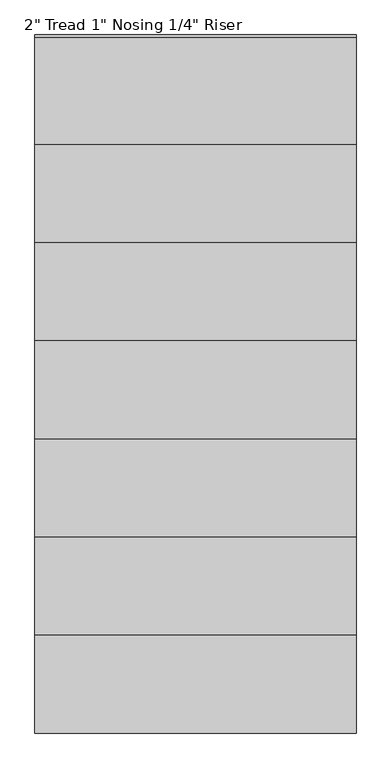
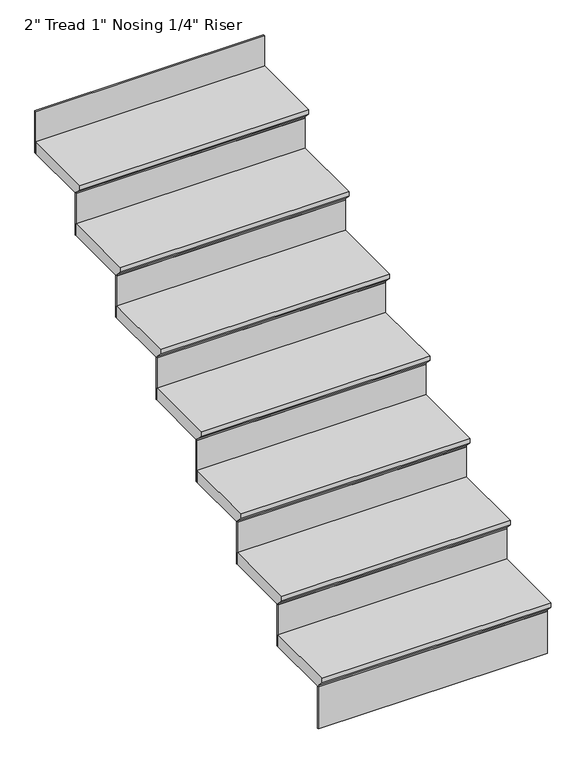
"""IFC4 building model written with IfcOpenShell, lengths in millimetres: stair flight geometry."""

from ifc_helpers import new_model, si_unit, frame, origin, place, context, project, spatial, polyline, outline, extrude, source, transform, mapped, element, save


def stair_flight_a0137449(model_context):
    return source(origin(), model_context, "Body", "SweptSolid", [
        extrude(outline(polyline([(-3589.3064015, 5765.8), (-3284.5064015, 5765.8), (-3284.5064015, 5715.0), (-3563.9064015, 5715.0), (-3563.9064015, 5721.35), (-3589.3064015, 5746.75), (-3589.3064015, 5765.8)])), frame((13296.7506237, 0.0, 0.0), z_axis=(1.0, 0.0, 0.0), x_axis=(0.0, 1.0, 0.0)), (0.0, 0.0, 1.0), 914.4),
        extrude(outline(polyline([(14211.1506237, -3557.5564015), (14211.1506237, -3563.9064015), (13296.7506237, -3563.9064015), (13296.7506237, -3557.5564015), (14211.1506237, -3557.5564015)])), frame((0.0, 0.0, 5537.2), z_axis=(0.0, 0.0, 1.0), x_axis=(1.0, 0.0, 0.0)), (0.0, 0.0, 1.0), 177.8),
        extrude(outline(polyline([(14211.1506237, -3278.1564015), (14211.1506237, -3284.5064015), (13296.7506237, -3284.5064015), (13296.7506237, -3278.1564015), (14211.1506237, -3278.1564015)])), frame((0.0, 0.0, 5715.0), z_axis=(0.0, 0.0, 1.0), x_axis=(1.0, 0.0, 0.0)), (0.0, 0.0, 1.0), 177.8),
        extrude(outline(polyline([(-3309.9064015, 5943.6), (-3005.1064015, 5943.6), (-3005.1064015, 5892.8), (-3284.5064015, 5892.8), (-3284.5064015, 5899.15), (-3309.9064015, 5924.55), (-3309.9064015, 5943.6)])), frame((13296.7506237, 0.0, 0.0), z_axis=(1.0, 0.0, 0.0), x_axis=(0.0, 1.0, 0.0)), (0.0, 0.0, 1.0), 914.4),
        extrude(outline(polyline([(14211.1506237, -2998.7564015), (14211.1506237, -3005.1064015), (13296.7506237, -3005.1064015), (13296.7506237, -2998.7564015), (14211.1506237, -2998.7564015)])), frame((0.0, 0.0, 5892.8), z_axis=(0.0, 0.0, 1.0), x_axis=(1.0, 0.0, 0.0)), (0.0, 0.0, 1.0), 177.8),
        extrude(outline(polyline([(-3030.5064015, 6121.4), (-2725.7064015, 6121.4), (-2725.7064015, 6070.6), (-3005.1064015, 6070.6), (-3005.1064015, 6076.95), (-3030.5064015, 6102.35), (-3030.5064015, 6121.4)])), frame((13296.7506237, 0.0, 0.0), z_axis=(1.0, 0.0, 0.0), x_axis=(0.0, 1.0, 0.0)), (0.0, 0.0, 1.0), 914.4),
        extrude(outline(polyline([(14211.1506237, -2719.3564015), (14211.1506237, -2725.7064015), (13296.7506237, -2725.7064015), (13296.7506237, -2719.3564015), (14211.1506237, -2719.3564015)])), frame((0.0, 0.0, 6070.6), z_axis=(0.0, 0.0, 1.0), x_axis=(1.0, 0.0, 0.0)), (0.0, 0.0, 1.0), 177.8),
        extrude(outline(polyline([(-2751.1064015, 6299.2), (-2446.3064015, 6299.2), (-2446.3064015, 6248.4), (-2725.7064015, 6248.4), (-2725.7064015, 6254.75), (-2751.1064015, 6280.15), (-2751.1064015, 6299.2)])), frame((13296.7506237, 0.0, 0.0), z_axis=(1.0, 0.0, 0.0), x_axis=(0.0, 1.0, 0.0)), (0.0, 0.0, 1.0), 914.4),
        extrude(outline(polyline([(14211.1506237, -2439.9564015), (14211.1506237, -2446.3064015), (13296.7506237, -2446.3064015), (13296.7506237, -2439.9564015), (14211.1506237, -2439.9564015)])), frame((0.0, 0.0, 6248.4), z_axis=(0.0, 0.0, 1.0), x_axis=(1.0, 0.0, 0.0)), (0.0, 0.0, 1.0), 177.8),
        extrude(outline(polyline([(-2471.7064015, 6477.0), (-2166.9064015, 6477.0), (-2166.9064015, 6426.2), (-2446.3064015, 6426.2), (-2446.3064015, 6432.55), (-2471.7064015, 6457.95), (-2471.7064015, 6477.0)])), frame((13296.7506237, 0.0, 0.0), z_axis=(1.0, 0.0, 0.0), x_axis=(0.0, 1.0, 0.0)), (0.0, 0.0, 1.0), 914.4),
        extrude(outline(polyline([(14211.1506237, -2160.5564015), (14211.1506237, -2166.9064015), (13296.7506237, -2166.9064015), (13296.7506237, -2160.5564015), (14211.1506237, -2160.5564015)])), frame((0.0, 0.0, 6426.2), z_axis=(0.0, 0.0, 1.0), x_axis=(1.0, 0.0, 0.0)), (0.0, 0.0, 1.0), 177.8),
        extrude(outline(polyline([(-2192.3064015, 6654.8), (-1887.5064015, 6654.8), (-1887.5064015, 6604.0), (-2166.9064015, 6604.0), (-2166.9064015, 6610.35), (-2192.3064015, 6635.75), (-2192.3064015, 6654.8)])), frame((13296.7506237, 0.0, 0.0), z_axis=(1.0, 0.0, 0.0), x_axis=(0.0, 1.0, 0.0)), (0.0, 0.0, 1.0), 914.4),
        extrude(outline(polyline([(14211.1506237, -1881.1564015), (14211.1506237, -1887.5064015), (13296.7506237, -1887.5064015), (13296.7506237, -1881.1564015), (14211.1506237, -1881.1564015)])), frame((0.0, 0.0, 6604.0), z_axis=(0.0, 0.0, 1.0), x_axis=(1.0, 0.0, 0.0)), (0.0, 0.0, 1.0), 177.8),
        extrude(outline(polyline([(14211.1506237, -1601.7564015), (14211.1506237, -1608.1064015), (13296.7506237, -1608.1064015), (13296.7506237, -1601.7564015), (14211.1506237, -1601.7564015)])), frame((0.0, 0.0, 6781.8), z_axis=(0.0, 0.0, 1.0), x_axis=(1.0, 0.0, 0.0)), (0.0, 0.0, 1.0), 177.8),
        extrude(outline(polyline([(-1912.9064015, 6832.6), (-1608.1064015, 6832.6), (-1608.1064015, 6781.8), (-1887.5064015, 6781.8), (-1887.5064015, 6788.15), (-1912.9064015, 6813.55), (-1912.9064015, 6832.6)])), frame((13296.7506237, 0.0, 0.0), z_axis=(1.0, 0.0, 0.0), x_axis=(0.0, 1.0, 0.0)), (0.0, 0.0, 1.0), 914.4),
    ])


if __name__ == "__main__":
    model = new_model("IFC4")
    model_context = context("Model", 3, world=origin())
    ifc_project = project(units=[si_unit("LENGTHUNIT", "METRE", prefix="MILLI")], contexts=[model_context])
    site = spatial("IfcSite", under=ifc_project)
    building = spatial("IfcBuilding", under=site)
    placement = place(None, origin())
    stair_flight_shape = stair_flight_a0137449(model_context)
    element("IfcStairFlight", 1, ObjectType="2\" Tread 1\" Nosing 1/4\" Riser", at=placement, inside=building, context=model_context, shape_type="MappedRepresentation", body=[
        mapped(stair_flight_shape, transform((0.0, 0.0, 0.0), x_axis=(1.0, 0.0, 0.0), y_axis=(0.0, 1.0, 0.0), z_axis=(0.0, 0.0, 1.0))),
    ])
    save(model, "model.ifc")
